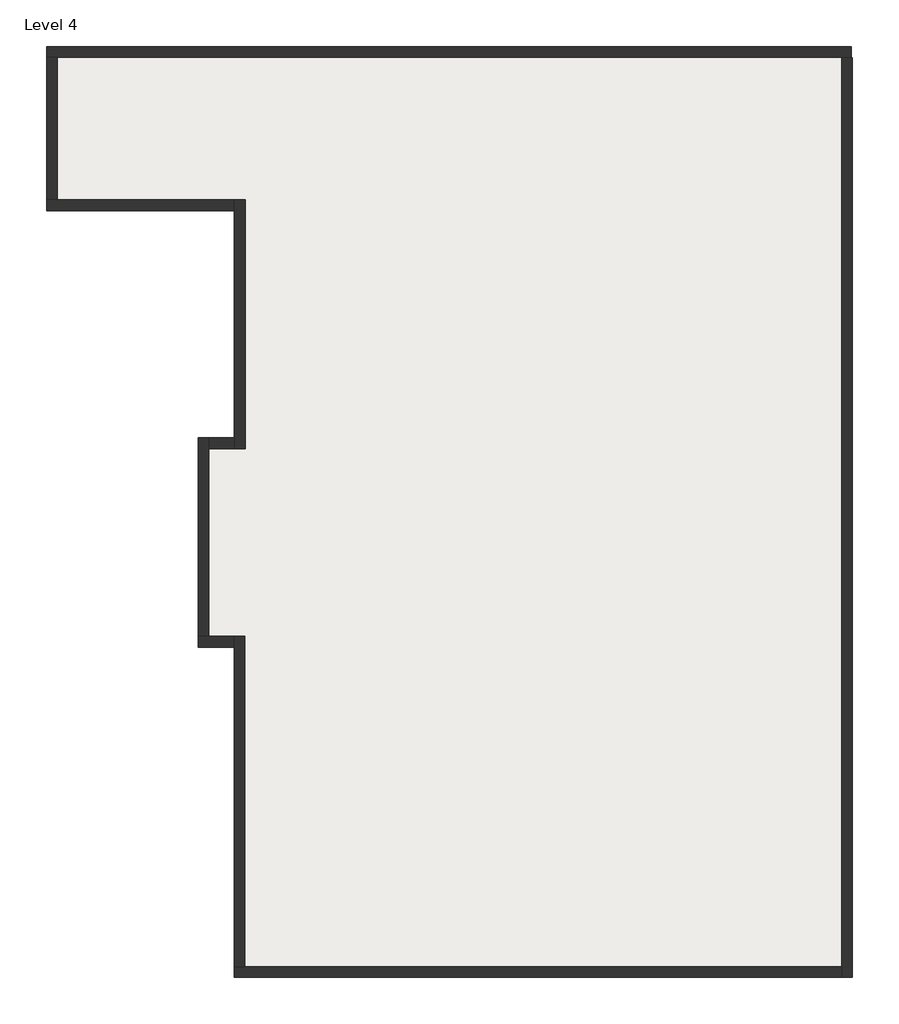
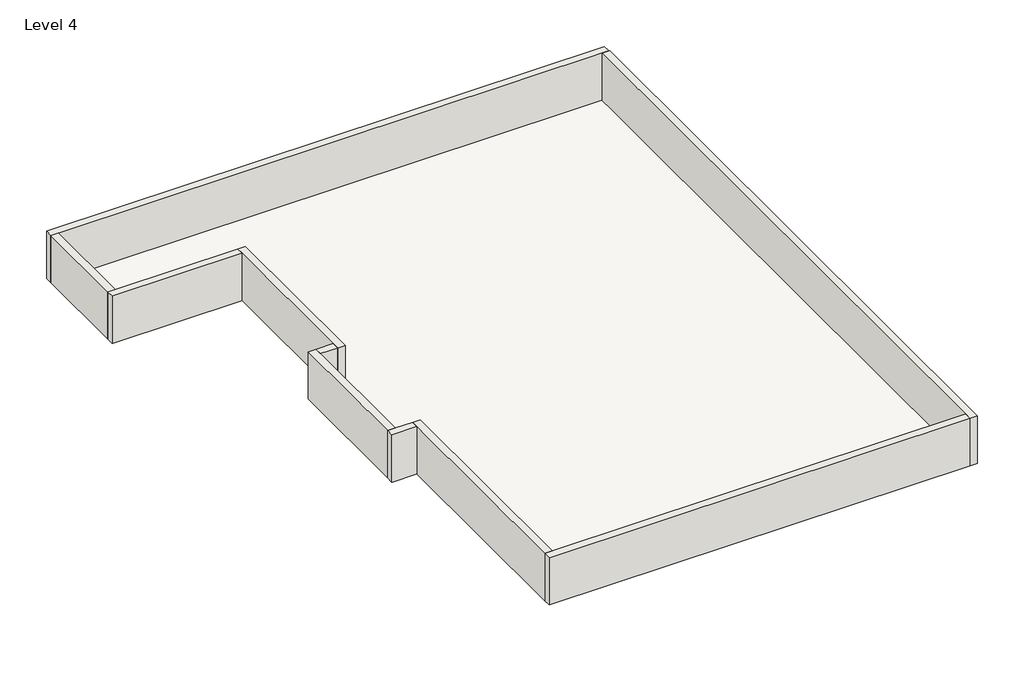
# One storey: 10 walls, 1 roof.
"""IFC4 building model written with IfcOpenShell, lengths in millimetres."""

from ifc_helpers import new_model, si_unit, frame, origin, place, context, project, spatial, polyline, outline, extrude, faceted_brep, element, save

model = new_model("IFC4")

# Units and contexts
model_context = context("Model", 3, world=origin())
ifc_project = project(units=[si_unit("LENGTHUNIT", "METRE", prefix="MILLI")], contexts=[model_context])

# Site, building, storey
site = spatial("IfcSite", under=ifc_project)
building = spatial("IfcBuilding", under=site)
storey = spatial("IfcBuildingStorey", under=building, Name="Level 4", Elevation=6400.8)

# Roof
placement = place(None, origin())
element("IfcRoof", 1, ObjectType="Generic - 12\"", at=placement, inside=storey, context=model_context, shape_type="SweptSolid", body=[
    extrude(outline(polyline([(-10241.6673123, 12262.9722985), (6410.607868, 12262.9722985), (6410.607868, -6937.6042186), (-6239.1057305, -6937.6042186), (-6239.1057305, 34.6957814), (-7000.592132, 34.6957814), (-7000.592132, 3997.0957814), (-6238.592132, 3997.0957814), (-6238.592132, 9214.9722985), (-10241.6673123, 9214.9722985), (-10241.6673123, 12262.9722985)])), frame((0.0, 0.0, 6248.4), z_axis=(0.0, 0.0, 1.0), x_axis=(1.0, 0.0, 0.0)), (0.0, 0.0, 1.0), 152.4),
])

# Walls
element("IfcWall", 2, ObjectType="WALL9\"", at=placement, inside=storey, context=model_context, shape_type="Brep", body=[
    faceted_brep([(-10429.592132, 12262.9722985, 6400.8), (-10200.992132, 12262.9722985, 6400.8), (6563.007868, 12262.9722985, 6400.8), (6563.007868, 12262.9722985, 7924.8), (-10200.992132, 12262.9722985, 7924.8), (-10429.592132, 12262.9722985, 7924.8), (-10429.592132, 12491.5722985, 6400.8), (-10429.592132, 12491.5722985, 7924.8), (6563.007868, 12491.5722985, 7924.8), (6563.007868, 12491.5722985, 6400.8)], [[[0, 1, 2, 3, 4, 5]], [[6, 7, 8, 9]], [[0, 5, 7, 6]], [[2, 1, 0, 6, 9]], [[3, 2, 9, 8]], [[5, 4, 3, 8, 7]]]),
])
element("IfcWall", 3, ObjectType="WALL9\"", at=placement, inside=storey, context=model_context, shape_type="Brep", body=[
    faceted_brep([(6359.807868, 12252.0957814, 6400.8), (6359.807868, -6937.6042186, 6400.8), (6359.807868, -7166.2042186, 6400.8), (6359.807868, -7166.2042186, 7924.8), (6359.807868, -6937.6042186, 7924.8), (6359.807868, 12252.0957814, 7924.8), (6588.407868, 12252.0957814, 6400.8), (6588.407868, 12252.0957814, 7924.8), (6588.407868, -7166.2042186, 7924.8), (6588.407868, -7166.2042186, 6400.8)], [[[0, 1, 2, 3, 4, 5]], [[6, 7, 8, 9]], [[2, 1, 0, 6, 9]], [[5, 4, 3, 8, 7]], [[0, 5, 7, 6]], [[3, 2, 9, 8]]]),
])
element("IfcWall", 4, ObjectType="WALL9\"", at=placement, inside=storey, context=model_context, shape_type="Brep", body=[
    faceted_brep([(6359.807868, -6937.6042186, 6400.8), (-6239.1057305, -6937.6042186, 6400.8), (-6467.7057305, -6937.6042186, 6400.8), (-6467.7057305, -6937.6042186, 7924.8), (-6239.1057305, -6937.6042186, 7924.8), (6359.807868, -6937.6042186, 7924.8), (6359.807868, -7166.2042186, 6400.8), (6359.807868, -7166.2042186, 7924.8), (-6467.7057305, -7166.2042186, 7924.8), (-6467.7057305, -7166.2042186, 6400.8)], [[[0, 1, 2, 3, 4, 5]], [[6, 7, 8, 9]], [[2, 1, 0, 6, 9]], [[5, 4, 3, 8, 7]], [[0, 5, 7, 6]], [[3, 2, 9, 8]]]),
])
element("IfcWall", 5, ObjectType="WALL9\"", at=placement, inside=storey, context=model_context, shape_type="Brep", body=[
    faceted_brep([(-6239.1057305, -6937.6042186, 6400.8), (-6239.1057305, 34.6957814, 6400.8), (-6239.1057305, 34.6957814, 7924.8), (-6239.1057305, -6937.6042186, 7924.8), (-6467.7057305, -6937.6042186, 6400.8), (-6467.7057305, -6937.6042186, 7924.8), (-6467.7057305, -193.9042186, 7924.8), (-6467.7057305, 34.6957814, 7924.8), (-6467.7057305, 34.6957814, 6400.8), (-6467.7057305, -193.9042186, 6400.8)], [[[0, 1, 2, 3]], [[4, 5, 6, 7, 8, 9]], [[1, 0, 4, 9, 8]], [[3, 2, 7, 6, 5]], [[0, 3, 5, 4]], [[2, 1, 8, 7]]]),
])
element("IfcWall", 6, ObjectType="WALL9\"", at=placement, inside=storey, context=model_context, shape_type="Brep", body=[
    faceted_brep([(-6467.7057305, 34.6957814, 6400.8), (-7000.592132, 34.6957814, 6400.8), (-7229.192132, 34.6957814, 6400.8), (-7229.192132, 34.6957814, 7924.8), (-7000.592132, 34.6957814, 7924.8), (-6467.7057305, 34.6957814, 7924.8), (-6467.7057305, -193.9042186, 6400.8), (-6467.7057305, -193.9042186, 7924.8), (-7229.192132, -193.9042186, 7924.8), (-7229.192132, -193.9042186, 6400.8)], [[[0, 1, 2, 3, 4, 5]], [[6, 7, 8, 9]], [[2, 1, 0, 6, 9]], [[5, 4, 3, 8, 7]], [[0, 5, 7, 6]], [[3, 2, 9, 8]]]),
])
element("IfcWall", 7, ObjectType="WALL9\"", at=placement, inside=storey, context=model_context, shape_type="Brep", body=[
    faceted_brep([(-7000.592132, 34.6957814, 6400.8), (-7000.592132, 3997.0957814, 6400.8), (-7000.592132, 4225.6957814, 6400.8), (-7000.592132, 4225.6957814, 7924.8), (-7000.592132, 3997.0957814, 7924.8), (-7000.592132, 34.6957814, 7924.8), (-7229.192132, 34.6957814, 6400.8), (-7229.192132, 34.6957814, 7924.8), (-7229.192132, 4225.6957814, 7924.8), (-7229.192132, 4225.6957814, 6400.8)], [[[0, 1, 2, 3, 4, 5]], [[6, 7, 8, 9]], [[2, 1, 0, 6, 9]], [[5, 4, 3, 8, 7]], [[0, 5, 7, 6]], [[3, 2, 9, 8]]]),
])
element("IfcWall", 8, ObjectType="WALL9\"", at=placement, inside=storey, context=model_context, shape_type="Brep", body=[
    faceted_brep([(-6238.592132, 3997.0957814, 6400.8), (-6238.592132, 9254.8957814, 6400.8), (-6238.592132, 9254.8957814, 7924.8), (-6238.592132, 3997.0957814, 7924.8), (-6467.192132, 3997.0957814, 6400.8), (-6467.192132, 3997.0957814, 7924.8), (-6467.192132, 4225.6957814, 7924.8), (-6467.192132, 9026.2957814, 7924.8), (-6467.192132, 9254.8957814, 7924.8), (-6467.192132, 9254.8957814, 6400.8), (-6467.192132, 9026.2957814, 6400.8), (-6467.192132, 4225.6957814, 6400.8)], [[[0, 1, 2, 3]], [[4, 5, 6, 7, 8, 9, 10, 11]], [[1, 0, 4, 11, 10, 9]], [[3, 2, 8, 7, 6, 5]], [[2, 1, 9, 8]], [[0, 3, 5, 4]]]),
])
element("IfcWall", 9, ObjectType="WALL9\"", at=placement, inside=storey, context=model_context, shape_type="Brep", body=[
    faceted_brep([(-6467.192132, 9254.8957814, 6400.8), (-10200.992132, 9254.8957814, 6400.8), (-10429.592132, 9254.8957814, 6400.8), (-10429.592132, 9254.8957814, 7924.8), (-10200.992132, 9254.8957814, 7924.8), (-6467.192132, 9254.8957814, 7924.8), (-6467.192132, 9026.2957814, 6400.8), (-6467.192132, 9026.2957814, 7924.8), (-10429.592132, 9026.2957814, 7924.8), (-10429.592132, 9026.2957814, 6400.8)], [[[0, 1, 2, 3, 4, 5]], [[6, 7, 8, 9]], [[2, 1, 0, 6, 9]], [[5, 4, 3, 8, 7]], [[0, 5, 7, 6]], [[3, 2, 9, 8]]]),
])
element("IfcWall", 10, ObjectType="WALL9\"", at=placement, inside=storey, context=model_context, shape_type="SweptSolid", body=[
    extrude(outline(polyline([(-10200.992132, 12262.9722985), (-10200.992132, 9254.8957814), (-10429.592132, 9254.8957814), (-10429.592132, 12262.9722985), (-10200.992132, 12262.9722985)])), frame((0.0, 0.0, 6400.8), z_axis=(0.0, 0.0, 1.0), x_axis=(1.0, 0.0, 0.0)), (0.0, 0.0, 1.0), 1524.0),
])
element("IfcWall", 11, ObjectType="WALL9\"", at=placement, inside=storey, context=model_context, shape_type="SweptSolid", body=[
    extrude(outline(polyline([(-6467.192132, 3997.0957814), (-7000.592132, 3997.0957814), (-7000.592132, 4225.6957814), (-6467.192132, 4225.6957814), (-6467.192132, 3997.0957814)])), frame((0.0, 0.0, 6400.8), z_axis=(0.0, 0.0, 1.0), x_axis=(1.0, 0.0, 0.0)), (0.0, 0.0, 1.0), 1524.0),
])

save(model, "model.ifc")

# Revit data of these elements
# Type "Generic - 12\""
#   Assembly Code = "B1020"
#   Layers, outside or top first: 0' - 6" no material (function 1)
# Type "WALL9\""
#   Assembly Code = "B2010"
#   Layers, outside or top first: 0' - 9" no material (function 1)
# Element 1 (IfcRoof, "Generic - 12\"")
#   built-in parameter 1001705 = 21 (stored number, unit not read)
#   built-in parameter 1001701 = -0.5 (stored number, unit not read)
#   built-in parameter 1001710 = 33615
#   Phase Created = New Construction
#   Materials on its faces: "Default Roof"
# Elements 2, 3, 4, 5, 6, 7, 8, 9, 10, 11 (IfcWall, "WALL9\"")
#   Top Offset = 0' - 0"
#   Base Offset = 0' - 0"
#   Unconnected Height = 5' - 0"
#   wall height = 5' - 0"
#   Phase Created = New Construction
#   Base Constraint = Level 4
#   Materials on its faces: "Default Wall"
# Materials
#   "Default Roof": colour RGB 88 101 114, transparency 0, Cost = 0
#   "Default Wall": colour RGB 128 128 128, transparency 0, Cost = 0
